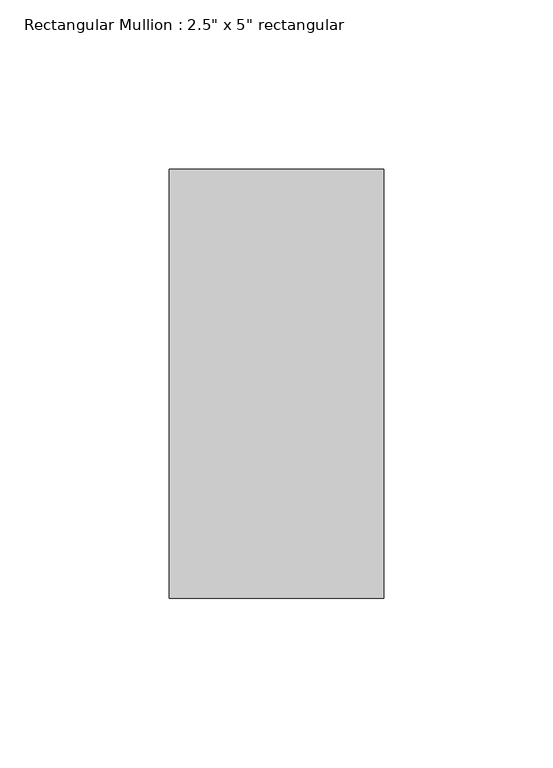
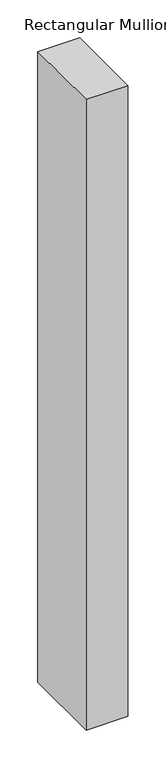
"""IFC4 building model written with IfcOpenShell, lengths in millimetres: member geometry."""

from ifc_helpers import new_model, si_unit, frame, origin, place, context, project, spatial, polyline, outline, extrude, source, transform, mapped, element, save


def member_8e09d03a(model_context):
    return source(origin(), model_context, "Body", "SweptSolid", [
        extrude(outline(polyline([(0.0, 63.5), (0.0, -63.5), (-63.5, -63.5), (-63.5, 63.5), (0.0, 63.5)])), frame((0.0, 0.0, -1016.0), z_axis=(0.0, 0.0, 1.0), x_axis=(1.0, 0.0, 0.0)), (0.0, 0.0, 1.0), 1016.0),
    ])


if __name__ == "__main__":
    model = new_model("IFC4")
    model_context = context("Model", 3, world=origin())
    ifc_project = project(units=[si_unit("LENGTHUNIT", "METRE", prefix="MILLI")], contexts=[model_context])
    site = spatial("IfcSite", under=ifc_project)
    building = spatial("IfcBuilding", under=site)
    placement = place(None, origin())
    member_shape = member_8e09d03a(model_context)
    element("IfcMember", 1, ObjectType="Rectangular Mullion : 2.5\" x 5\" rectangular", at=placement, inside=building, context=model_context, shape_type="MappedRepresentation", body=[
        mapped(member_shape, transform((0.0, 0.0, 0.0), x_axis=(1.0, 0.0, 0.0), y_axis=(0.0, 1.0, 0.0), z_axis=(0.0, 0.0, 1.0))),
    ])
    save(model, "model.ifc")

# Revit data of these elements
# Type "Rectangular Mullion : 2.5\" x 5\" rectangular"
#   built-in parameter 1007304 = 0.416667 (stored number, unit not read)
#   built-in parameter 1007301 = 0.104167 (stored number, unit not read)
#   built-in parameter 1007300 = 0.104167 (stored number, unit not read)
# Element 1 (IfcMember, "Rectangular Mullion : 2.5\" x 5\" rectangular")
#   Materials on its faces: "Aluminum"
# Materials
#   "Aluminum": class "Metal", colour RGB 247 247 247, transparency 0, Description = "Aluminum 6061", Cost = 0
